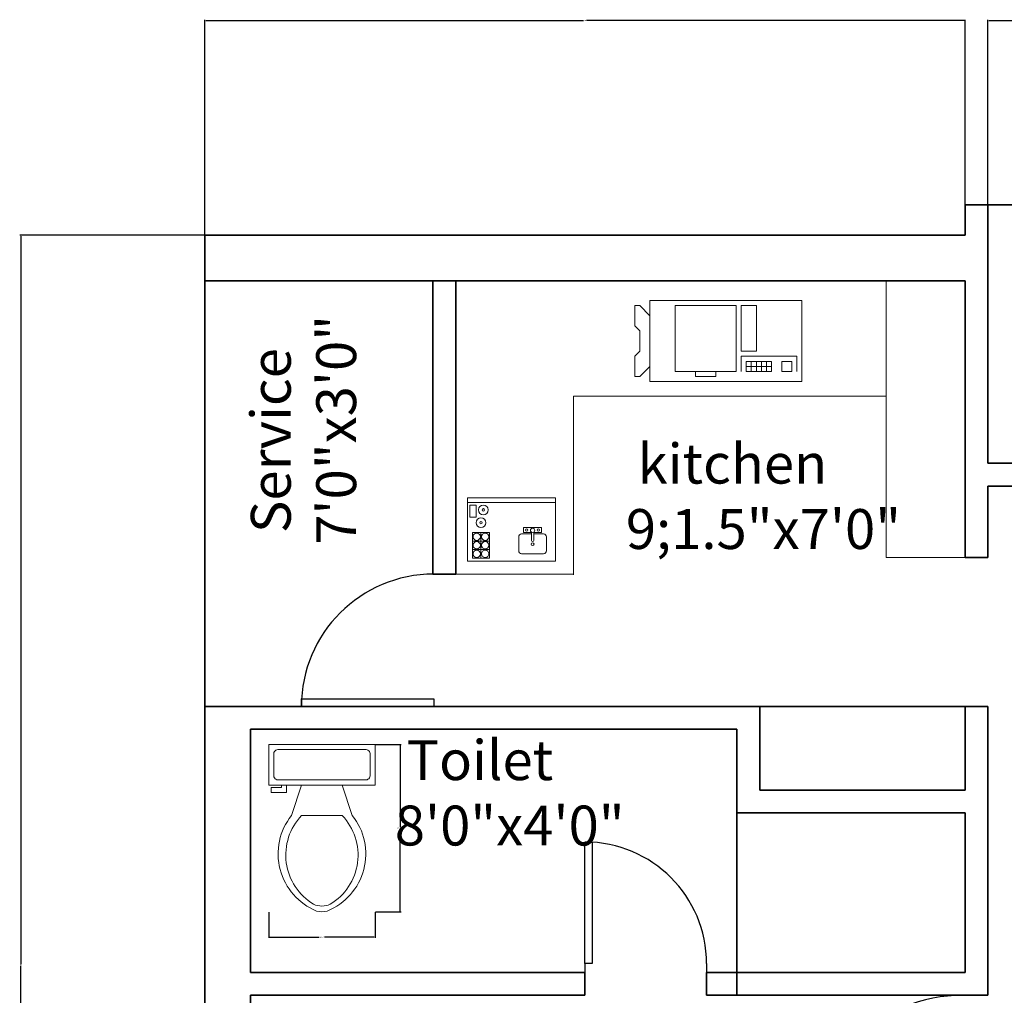
# Model space of a CAD drawing. Units: inches. Extents: x 108 to 613, y 1573 to 2319.
# Tile 8 of 11: x 108 to 303, y 2127 to 2319. Entities that reach past the tile are written whole.
import ezdxf

# ---------------------------------------------------------------- set-up
doc = ezdxf.new("R2010")
doc.units = ezdxf.units.IN
for name, color, linetype, lineweight in [('A-ANNO-DIMS', 2, 'Continuous', 18), ('A-AREA-IDEN', 3, 'Continuous', 18), ('A-EQPM', 2, 'Continuous', 18), ('A-FLOR-CASE', 6, 'Continuous', 18), ('A-FLOR-FIXT', 2, 'Continuous', 18), ('door', 4, 'Continuous', 25), ('wall', 6, 'Continuous', 35)]:
    doc.layers.add(name, color=color, linetype=linetype, lineweight=lineweight)
doc.styles.get("Standard").update_dxf_attribs({"font": 'arial.ttf'})
doc.dimstyles.get("Standard").update_dxf_attribs({"dimtxt": 0.18, "dimasz": 0.18, "dimexe": 0.18, "dimexo": 0.0625, "dimgap": 0.09, "dimtad": 0, "dimtih": 1, "dimtoh": 1, "dimdec": 4, "dimzin": 0, "dimdsep": 46, "dimtxsty": 'Standard', "dimcen": 0.09, "dimadec": 0, "dimazin": 0, "dimtfac": 1, "dimtdec": 4, "dimtofl": 0, "dimtmove": 0, "dimatfit": 3, "dimfxl": 1, "dimtolj": 1, "dimtzin": 0, "dimarcsym": 0})

# ---------------------------------------------------------------- blocks, each defined once
blk = doc.blocks.new('*U2')
for p, q in [((0, 0), (0, -5)), ((30, 0), (30, -5))]:
    blk.add_line(p, q)
blk.add_lwpolyline([(0, 0), (0, 30), (1.75, 30), (1.75, 0)], close=True)
blk.add_arc((0, 0), 30, 0, 90)
blk = doc.blocks.new('Copy Machine')
for p, q in [((0, 0), (0, -16)), ((30, 0), (0, 0)), ((30, -16), (30, 0)), ((-3, -1), (-3, -5)), ((-2, -1), (-3, -1)), ((0, -3), (-2, -1)), ((5, -1), (5, -14)), ((17, -1), (5, -1)), ((17, -14), (17, -1)), ((18, -1), (18, -10)), ((21, -1), (18, -1)), ((21, -10), (21, -1)), ((-3, -5), (-2, -6)), ((-2, -10), (-2, -6)), ((-3, -11), (-2, -10)), ((-3, -15), (-3, -11)), ((18, -10), (21, -10)), ((18, -14), (18, -11)), ((18, -11), (29, -11)), ((29, -11), (29, -14)), ((0, -13), (-2, -15)), ((24, -12), (19, -12)), ((19, -12), (19, -14)), ((24, -13), (19, -13)), ((20, -12), (20, -14)), ((21, -14), (21, -12)), ((22, -12), (22, -14)), ((23, -14), (23, -12)), ((24, -14), (24, -12)), ((28, -12), (26, -12)), ((26, -12), (26, -14)), ((28, -14), (28, -12)), ((-2, -15), (-3, -15)), ((5, -14), (17, -14)), ((9, -14), (9, -15)), ((9, -15), (13, -15)), ((13, -15), (13, -14)), ((19, -14), (24, -14)), ((26, -14), (28, -14)), ((0, -16), (30, -16))]:
    blk.add_line(p, q)
blk = doc.blocks.new('Wet Bar')
for p, q in [((0, 0), (36, 0)), ((0, -26), (0, 0)), ((36, 0), (36, -26)), ((0, -2), (36, -2)), ((3.5, -3), (1, -3)), ((1, -3), (1, -8)), ((3.5, -8), (3.5, -3)), ((1, -8), (3.5, -8)), ((2, -14.25), (9, -14.25)), ((2, -24.75), (2, -14.25)), ((5.5, -14.25), (5.5, -24.75)), ((9, -14.25), (9, -24.75)), ((26.2, -17.55), (26.2, -14.1284)), ((27.1001, -17.55), (27.1001, -14.1284)), ((2, -17.75), (9, -17.75)), ((9, -21.25), (2, -21.25)), ((36, -26), (0, -26)), ((9, -24.75), (2, -24.75))]:
    blk.add_line(p, q)
for points in [[(20.95, -21.75), (20.95, -16.05)], [(22.15, -14.85), (26.2, -14.85)], [(26.2, -14.25), (22.95, -14.25), (22.95, -12.2), (26.75, -12.2)], [(26.7487, -12.2), (30.3501, -12.2), (30.3501, -14.25), (27.1001, -14.25)], [(27.1001, -14.85), (31.15, -14.85)], [(32.3501, -16.05), (32.3501, -21.75)], [(31.15, -22.95), (22.15, -22.95)]]:
    blk.add_lwpolyline(points)
for centre, radius in [((6.5, -5), 2), ((6.5, -5), 0.5), ((5.5, -10.25), 2), ((5.5, -10.25), 0.5), ((3.75, -16), 1.5), ((7.25, -16), 1.5), ((24.25, -13.25), 0.5), ((26.65, -13.35), 0.9), ((29, -13.25), 0.5), ((3.75, -19.5), 1.5), ((7.25, -19.5), 1.5), ((26.65, -19.05), 0.6), ((3.75, -23), 1.5), ((7.25, -23), 1.5)]:
    blk.add_circle(centre, radius)
for centre, radius, start, end in [((22.2251, -16.125), 1.2772, 93.36646, 176.6335), ((31.075, -16.125), 1.2772, 3.366461, 86.63354), ((26.65, -17.55), 0.45, 180, 0), ((22.2251, -21.675), 1.2772, 183.3665, 266.6335), ((31.075, -21.675), 1.2772, 273.3665, 356.6335)]:
    blk.add_arc(centre, radius, start, end)
blk = doc.blocks.new('Toilet - top')
for p, q in [((9.5, -6), (9.5, -2)), ((-10, -8.5), (-8, -8.5)), ((-10, -9.5), (-10, -8.5)), ((-7, -9.5), (-10, -9.5)), ((-8, -8.5), (-8, -8)), ((-7, -8), (-7, -9.5)), ((-4, -8), (-6, -14)), ((4, -8), (6, -14)), ((4, -14), (-4, -14))]:
    blk.add_line(p, q)
blk.add_lwpolyline([(10.5, -8), (10.5, 0), (-10.5, 0), (-10.5, -8)], close=True)
for points in [[(8.5, -1), (-8.5, -1)], [(-9.5, -2), (-9.5, -6)], [(-8.5, -7), (8.5, -7)]]:
    blk.add_lwpolyline(points)
for centre, radius, start, end in [((-8.62, -1.88), 0.884, 81.8699, 188.1301), ((8.62, -1.88), 0.884, 351.8699, 98.1301), ((-8.62, -6.12), 0.884, 171.8699, 278.1301), ((8.62, -6.12), 0.884, 261.8699, 8.1301), ((3.52, -21.58), 12.17, 141.4691, 247.9714), ((4.2, -21.82), 11.33, 136.3677, 238.9468), ((-3.52, -21.58), 12.17, 292.0284, 38.5307), ((-4.2, -21.82), 11.33, 301.053, 43.6321), ((0, -27.88), 4, 245.7318, 294.2682), ((0, -29), 4, 254.8605, 285.1395)]:
    blk.add_arc(centre, radius, start, end)
blk = doc.blocks.new('*D23')
at = {"layer": 'A-ANNO-DIMS', "color": 0, "lineweight": -2, "transparency": 16777216}
for p, q in [((178.43, 2176.11), (183.5, 2176.11)), ((183.32, 2175.93), (183.32, 2159.77)), ((183.32, 2143.24), (183.32, 2159.4)), ((178.43, 2143.06), (183.5, 2143.06))]:
    blk.add_line(p, q, dxfattribs=at)
at = {"layer": 'A-ANNO-DIMS', "color": 0, "transparency": 16777216}
for points in [[(183.29, 2175.93), (183.35, 2175.93), (183.32, 2176.11)], [(183.29, 2143.24), (183.35, 2143.24), (183.32, 2143.06)]]:
    blk.add_solid(points, dxfattribs=at)
at = {"layer": 'Defpoints', "color": 0, "transparency": 16777216}
for p in [(178.36, 2176.11), (183.32, 2176.11), (178.36, 2143.06)]:
    blk.add_point(p, dxfattribs=at)
at = {"layer": 'A-ANNO-DIMS', "color": 0, "transparency": 16777216, "insert": (183.32, 2159.59), "char_height": 0.18, "attachment_point": 5}
blk.add_mtext('\\A1;WC 33 TYP.', dxfattribs=at)
blk = doc.blocks.new('*D24')
at = {"layer": 'A-ANNO-DIMS', "color": 0, "lineweight": -2, "transparency": 16777216}
for p, q in [((157.36, 2143), (157.36, 2137.93)), ((178.36, 2143), (178.36, 2137.93)), ((157.54, 2138.11), (167.33, 2138.11)), ((178.18, 2138.11), (168.39, 2138.11))]:
    blk.add_line(p, q, dxfattribs=at)
at = {"layer": 'A-ANNO-DIMS', "color": 0, "transparency": 16777216}
for points in [[(157.54, 2138.14), (157.54, 2138.08), (157.36, 2138.11)], [(178.18, 2138.14), (178.18, 2138.08), (178.36, 2138.11)]]:
    blk.add_solid(points, dxfattribs=at)
at = {"layer": 'Defpoints', "color": 0, "transparency": 16777216}
for p in [(157.36, 2143.06), (178.36, 2143.06), (178.36, 2138.11)]:
    blk.add_point(p, dxfattribs=at)
at = {"layer": 'A-ANNO-DIMS', "color": 0, "transparency": 16777216, "insert": (167.86, 2138.11), "char_height": 0.18, "attachment_point": 5}
blk.add_mtext('\\A1;21 TYP.', dxfattribs=at)
blk = doc.blocks.new('*D41')
at = {"layer": 'A-ANNO-DIMS', "color": 0, "lineweight": -2, "transparency": 16777216}
for p, q in [((144.78, 2276.67), (144.78, 2319.14)), ((144.96, 2318.96), (219.5, 2318.96)), ((294.6, 2318.96), (220.06, 2318.96)), ((294.78, 2282.67), (294.78, 2319.14))]:
    blk.add_line(p, q, dxfattribs=at)
at = {"layer": 'A-ANNO-DIMS', "color": 0, "transparency": 16777216}
for points in [[(144.96, 2318.99), (144.96, 2318.93), (144.78, 2318.96)], [(294.6, 2318.99), (294.6, 2318.93), (294.78, 2318.96)]]:
    blk.add_solid(points, dxfattribs=at)
at = {"layer": 'Defpoints', "color": 0, "transparency": 16777216}
for p in [(294.78, 2318.96), (294.78, 2282.61), (144.78, 2276.61)]:
    blk.add_point(p, dxfattribs=at)
at = {"layer": 'A-ANNO-DIMS', "color": 0, "transparency": 16777216, "insert": (219.78, 2318.96), "char_height": 0.18, "attachment_point": 5}
blk.add_mtext('\\A1;150', dxfattribs=at)
blk = doc.blocks.new('*D45')
at = {"layer": 'A-ANNO-DIMS', "color": 0, "lineweight": -2, "transparency": 16777216}
for p, q in [((144.71, 2276.61), (108.25, 2276.61)), ((108.43, 2276.43), (108.43, 2132.79)), ((108.43, 1988.79), (108.43, 2132.43)), ((144.71, 1988.61), (108.25, 1988.61))]:
    blk.add_line(p, q, dxfattribs=at)
at = {"layer": 'A-ANNO-DIMS', "color": 0, "transparency": 16777216}
for points in [[(108.4, 2276.43), (108.46, 2276.43), (108.43, 2276.61)], [(108.4, 1988.79), (108.46, 1988.79), (108.43, 1988.61)]]:
    blk.add_solid(points, dxfattribs=at)
at = {"layer": 'Defpoints', "color": 0, "transparency": 16777216}
for p in [(108.43, 2276.61), (144.78, 2276.61), (144.78, 1988.61)]:
    blk.add_point(p, dxfattribs=at)
at = {"layer": 'A-ANNO-DIMS', "color": 0, "transparency": 16777216, "insert": (108.43, 2132.61), "char_height": 0.18, "attachment_point": 5}
blk.add_mtext('\\A1;288', dxfattribs=at)
blk = doc.blocks.new('*D47')
at = {"layer": 'A-ANNO-DIMS', "color": 0, "lineweight": -2, "transparency": 16777216}
for p, q in [((299.28, 2231.67), (299.28, 2319.14)), ((299.46, 2318.96), (317.7, 2318.96)), ((336.6, 2318.96), (318.35, 2318.96)), ((336.78, 2231.67), (336.78, 2319.14))]:
    blk.add_line(p, q, dxfattribs=at)
at = {"layer": 'A-ANNO-DIMS', "color": 0, "transparency": 16777216}
for points in [[(299.46, 2318.99), (299.46, 2318.93), (299.28, 2318.96)], [(336.6, 2318.99), (336.6, 2318.93), (336.78, 2318.96)]]:
    blk.add_solid(points, dxfattribs=at)
at = {"layer": 'Defpoints', "color": 0, "transparency": 16777216}
for p in [(336.78, 2318.96), (299.28, 2231.61), (336.78, 2231.61)]:
    blk.add_point(p, dxfattribs=at)
at = {"layer": 'A-ANNO-DIMS', "color": 0, "transparency": 16777216, "insert": (318.03, 2318.96), "char_height": 0.18, "attachment_point": 5}
blk.add_mtext('\\A1;37.5', dxfattribs=at)

msp = doc.modelspace()

# ---------------------------------------------------------------- linework, layer by layer
at = {"layer": 'A-FLOR-CASE'}
for p, q in [((279.2445, 2247.2908), (279.2445, 2267.6125)), ((279.2445, 2267.6125), (279.2445, 2212.9845)), ((217.5399, 2209.577), (217.5399, 2244.8661)), ((217.5399, 2244.8661), (279.2445, 2244.8661)), ((279.2445, 2212.9845), (294.7753, 2212.9845)), ((217.5399, 2209.7306), (194.2753, 2209.7306))]:
    msp.add_line(p, q, dxfattribs=at)
at = {"layer": 'wall'}
for p, q in [((294.7753, 2282.6125), (294.7753, 2276.6125)), ((294.7753, 2282.6125), (435.7753, 2282.6125)), ((299.2753, 2282.6125), (299.2753, 2231.6125)), ((144.7753, 2276.6125), (144.7753, 1988.6125)), ((144.7753, 2276.6125), (294.7753, 2276.6125)), ((144.7753, 2267.6125), (294.7753, 2267.6125)), ((189.7753, 2267.6125), (189.7753, 2209.7306)), ((194.2753, 2267.6125), (194.2753, 2209.7306)), ((294.7753, 2267.6125), (294.7753, 2212.9845)), ((299.2753, 2231.6125), (336.7753, 2231.6125)), ((299.2753, 2227.1125), (336.7753, 2227.1125)), ((299.2753, 2227.1125), (299.2753, 2212.9845)), ((294.7753, 2212.9845), (299.2753, 2212.9845)), ((194.2753, 2209.7306), (189.7753, 2209.7306)), ((144.7753, 2183.6125), (254.2753, 2183.6125)), ((194.2753, 2183.6125), (299.2753, 2183.6125)), ((254.2753, 2183.6125), (254.2753, 2167.1125)), ((294.7753, 2183.6125), (294.7753, 2167.1125)), ((299.2753, 2183.6125), (299.2753, 2126.6125)), ((153.7753, 2179.1125), (249.7753, 2179.1125)), ((153.7753, 2179.1125), (153.7753, 2131.1125)), ((249.7753, 2179.1125), (249.7753, 2126.6125)), ((254.2753, 2167.1125), (294.7753, 2167.1125)), ((249.7753, 2162.6125), (294.7753, 2162.6125)), ((294.7753, 2162.6125), (294.7753, 2131.1125)), ((153.7753, 2131.1125), (219.7753, 2131.1125)), ((219.7753, 2131.1125), (219.7753, 2126.6125)), ((243.7753, 2131.1125), (243.7753, 2126.6125)), ((243.7753, 2131.1125), (294.7753, 2131.1125)), ((153.7753, 2126.6125), (219.7753, 2126.6125)), ((153.7753, 2126.6125), (153.7753, 1997.6125)), ((243.7753, 2126.6125), (299.2753, 2126.6125))]:
    msp.add_line(p, q, dxfattribs=at)

# ---------------------------------------------------------------- block references
at = {"layer": 'A-EQPM'}
msp.add_blockref('Copy Machine', (232.5992, 2263.7111), dxfattribs=at)
at = {"layer": 'A-FLOR-FIXT', "xscale": 0.4817065936809276, "yscale": 0.4817065936809276, "zscale": 0.4817065936809276}
msp.add_blockref('Wet Bar', (196.6022, 2224.8158), dxfattribs=at)
at = {"layer": 'A-FLOR-FIXT'}
msp.add_blockref('Toilet - top', (167.8631, 2176.1098), dxfattribs=at)
at = {"layer": 'door', "xscale": 0.870603593816971, "yscale": 0.870603593816971, "zscale": 0.870603593816971, "rotation": 89.99999999999991}
msp.add_blockref('*U2', (189.9223, 2183.6125), dxfattribs=at)
at = {"layer": 'door', "xscale": 0.8, "yscale": 0.8, "zscale": 0.8}
msp.add_blockref('*U2', (219.7753, 2132.8625), dxfattribs=at)
at = {"layer": 'door', "rotation": 89.99999999999991}
msp.add_blockref('*U2', (294.2753, 2096.6125), dxfattribs=at)

# ---------------------------------------------------------------- texts
at = {"layer": 'A-AREA-IDEN'}
for s, p in [('7\'0"x3\'0"', (174.6197, 2215.5221)), ('Service', (161.7138, 2217.8305))]:
    msp.add_text(s, height=7.87346, rotation=90, dxfattribs=at).set_placement(p)
for s, height, p in [('kitchen', 7.87346, (230.1554, 2227.5952)), ('9;1.5"x7\'0"', 7.873465, (227.847, 2214.6893)), ('Toilet', 7.87346, (184.5512, 2169.0831)), ('8\'0"x4\'0"', 7.87346, (182.2429, 2156.1772))]:
    msp.add_text(s, height=height, dxfattribs=at).set_placement(p)

# ---------------------------------------------------------------- dimensions: what is measured, and where the dimension line sits
at = {"layer": 'A-ANNO-DIMS'}
for base, p1, p2, override, picture, middle in [((294.7753, 2318.9625), (144.7753, 2276.6125), (294.7753, 2282.6125), {"dimdec": 0, "dimlfac": 1, "dimrnd": 0, "dimzin": 0, "dimdsep": 46, "dimlunit": 2}, '*D41', (219.7753, 2318.9625)), ((336.7753, 2318.9625), (299.2753, 2231.6125), (336.7753, 2231.6125), {"dimdec": 1, "dimlfac": 1, "dimrnd": 0, "dimzin": 0, "dimdsep": 46, "dimlunit": 2}, '*D47', (318.0253, 2318.9625))]:
    dim = msp.add_linear_dim(base=base, p1=p1, p2=p2, dimstyle='Standard', override=override, dxfattribs=at)
    dim.commit()
    dim.dimension.update_dxf_attribs({"geometry": picture, "text_midpoint": middle})
dim = msp.add_linear_dim(base=(108.4253, 2276.6125), p1=(144.7753, 1988.6125), p2=(144.7753, 2276.6125), angle=90, dimstyle='Standard', override={"dimdec": 0, "dimlfac": 1, "dimrnd": 0, "dimzin": 0, "dimdsep": 46, "dimlunit": 2}, dxfattribs=at)
dim.commit()
dim.dimension.update_dxf_attribs({"geometry": '*D45', "text_midpoint": (108.4253, 2132.6125)})
dim = msp.add_linear_dim(base=(183.32, 2176.1098), p1=(178.3631, 2143.0635), p2=(178.3631, 2176.1098), angle=90, text='WC <> TYP.', dimstyle='Standard', override={"dimdec": 0, "dimlfac": 1, "dimrnd": 0, "dimzin": 0, "dimdsep": 46, "dimlunit": 2}, dxfattribs=at)
dim.commit()
dim.dimension.update_dxf_attribs({"geometry": '*D23', "text_midpoint": (183.32, 2159.5867)})
dim = msp.add_linear_dim(base=(178.3631, 2138.1066), p1=(157.3631, 2143.0635), p2=(178.3631, 2143.0635), text='<> TYP.', dimstyle='Standard', override={"dimdec": 0, "dimlfac": 1, "dimrnd": 0, "dimzin": 0, "dimdsep": 46, "dimlunit": 2}, dxfattribs=at)
dim.commit()
dim.dimension.update_dxf_attribs({"geometry": '*D24', "text_midpoint": (167.8631, 2138.1066)})

doc.saveas('drawing.dxf')
